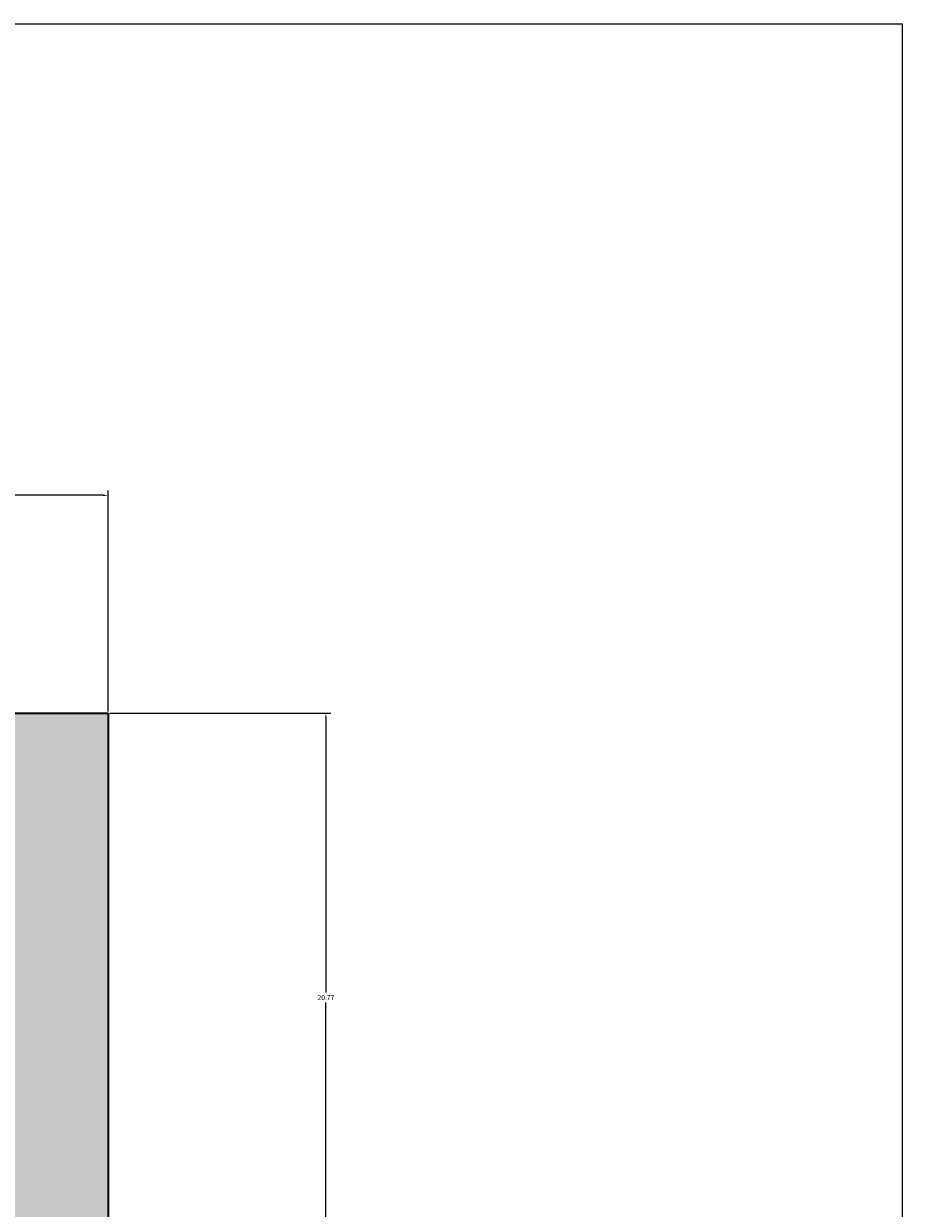
# Model space of a CAD drawing. Units: inches. Extents: x 4508 to 4723, y 847 to 1020.
# Tile 32 of 32: x 4691 to 4723, y 977 to 1020. Entities that reach past the tile are written whole.
import ezdxf

# ---------------------------------------------------------------- set-up
doc = ezdxf.new("R2010")
doc.units = ezdxf.units.IN
for name, color, linetype, lineweight in [('A-ANNO-DIMS', 2, 'Continuous', 18), ('A-ANNO-TTLB', 7, 'Continuous', 25), ('A-WALL', 7, 'Continuous', 35), ('A-WALL-PATT', 254, 'Continuous', 13)]:
    doc.layers.add(name, color=color, linetype=linetype, lineweight=lineweight)
doc.styles.get("Standard").update_dxf_attribs({"font": 'arial.ttf'})
doc.dimstyles.get("Standard").update_dxf_attribs({"dimtxt": 0.18, "dimasz": 0.18, "dimexe": 0.18, "dimexo": 0.0625, "dimgap": 0.09, "dimtad": 0, "dimtih": 1, "dimtoh": 1, "dimdec": 4, "dimzin": 0, "dimdsep": 46, "dimtxsty": 'Standard', "dimcen": 0.09, "dimadec": 0, "dimazin": 0, "dimtfac": 1, "dimtdec": 4, "dimtofl": 0, "dimtmove": 0, "dimatfit": 3, "dimfxl": 1, "dimtolj": 1, "dimtzin": 0, "dimarcsym": 0})

# ---------------------------------------------------------------- blocks, each defined once
blk = doc.blocks.new('*D11')
at = {"layer": 'A-ANNO-DIMS', "color": 0, "lineweight": -2, "transparency": 16777216}
for p, q in [((4671.806, 994.809), (4671.806, 1002.877)), ((4693.994, 994.809), (4693.994, 1002.877)), ((4671.986, 1002.697), (4682.435, 1002.697)), ((4693.814, 1002.697), (4683.365, 1002.697))]:
    blk.add_line(p, q, dxfattribs=at)
at = {"layer": 'A-ANNO-DIMS', "color": 0, "lineweight": 9, "transparency": 16777216}
for points in [[(4671.986, 1002.727), (4671.986, 1002.667), (4671.806, 1002.697)], [(4693.814, 1002.727), (4693.814, 1002.667), (4693.994, 1002.697)]]:
    blk.add_solid(points, dxfattribs=at)
at = {"layer": 'Defpoints', "color": 0, "lineweight": 9, "transparency": 16777216}
for p in [(4693.994, 1002.697), (4671.806, 994.747), (4693.994, 994.747)]:
    blk.add_point(p, dxfattribs=at)
at = {"layer": 'A-ANNO-DIMS', "color": 0, "transparency": 16777216, "insert": (4682.9, 1002.697), "char_height": 0.18, "attachment_point": 5}
blk.add_mtext('\\A1;22.188', dxfattribs=at)
blk = doc.blocks.new('*D23')
at = {"layer": 'A-ANNO-DIMS', "color": 0, "lineweight": -2, "transparency": 16777216}
for p, q in [((4694.056, 994.747), (4702.124, 994.747)), ((4701.944, 994.567), (4701.944, 984.545)), ((4701.944, 974.158), (4701.944, 984.181)), ((4669.387, 973.978), (4702.124, 973.978))]:
    blk.add_line(p, q, dxfattribs=at)
at = {"layer": 'A-ANNO-DIMS', "color": 0, "lineweight": 9, "transparency": 16777216}
for points in [[(4701.914, 994.567), (4701.974, 994.567), (4701.944, 994.747)], [(4701.914, 974.158), (4701.974, 974.158), (4701.944, 973.978)]]:
    blk.add_solid(points, dxfattribs=at)
at = {"layer": 'Defpoints', "color": 0, "lineweight": 9, "transparency": 16777216}
for p in [(4693.994, 994.747), (4701.944, 994.747), (4669.325, 973.978)]:
    blk.add_point(p, dxfattribs=at)
at = {"layer": 'A-ANNO-DIMS', "color": 0, "transparency": 16777216, "insert": (4701.944, 984.363), "char_height": 0.18, "attachment_point": 5}
blk.add_mtext('\\A1;20.77', dxfattribs=at)

msp = doc.modelspace()

# ---------------------------------------------------------------- hatches: boundary and pattern name
at = {"layer": 'A-WALL-PATT', "transparency": 33554508}
h = msp.add_hatch(color=256, dxfattribs=at)
h.dxf.hatch_style = 1
h.paths.add_polyline_path([(4661.6706, 954.043, -0.3739004), (4658.5765, 957.6021, -1), (4665.7646, 957.6021, -0.3739004), (4662.6706, 954.043), (4662.6706, 944.4021, -0.2114781), (4670.3062, 945.0869), (4670.3062, 968.0592, -0.4632086), (4663.3246, 973.9783, -0.4632086), (4670.3062, 979.8975), (4670.3062, 994.7469), (4588.9938, 994.7469), (4588.9938, 904.7469), (4657.9938, 904.7469), (4657.9938, 886.7469), (4549.9938, 886.7469), (4549.9938, 878.7469), (4693.9938, 878.7469), (4693.9938, 994.7469), (4671.8062, 994.7469), (4671.8062, 979.4411, -0.2941682), (4675.3246, 973.9783, -0.2941682), (4671.8062, 968.5156), (4671.8062, 944.4278, -0.2741114), (4676.7298, 936.1217, -0.2741114), (4671.8062, 927.8155), (4671.8062, 907.6998, -0.3779645), (4677.0562, 901.7469, -0.3779645), (4671.8062, 895.7939), (4671.8062, 883.7469), (4670.3062, 883.7469), (4670.3062, 895.7939, -0.3779645), (4665.0562, 901.7469, -0.3779645), (4670.3062, 907.6998), (4670.3062, 927.1564, -0.2114781), (4662.6706, 927.8412), (4662.6706, 918.2003, -0.3739004), (4665.7646, 914.6412, -1), (4658.5765, 914.6412, -0.3739004), (4661.6706, 918.2003), (4661.6706, 928.4807, -0.2391825), (4657.7936, 936.1217, -0.2391825), (4661.6706, 943.7626)])

# ---------------------------------------------------------------- linework, layer by layer
at = {"layer": 'A-ANNO-TTLB'}
msp.add_lwpolyline([(4508.3867, 1019.9118), (4722.9774, 1019.9118), (4722.9774, 846.9535), (4508.3867, 846.9535)], close=True, dxfattribs=at)
at = {"layer": 'A-WALL'}
for p, q in [((4540.9938, 994.7469), (4693.9938, 994.7469)), ((4693.9938, 994.7469), (4693.9938, 874.7469))]:
    msp.add_line(p, q, dxfattribs=at)

# ---------------------------------------------------------------- dimensions: what is measured, and where the dimension line sits
at = {"layer": 'A-ANNO-DIMS'}
dim = msp.add_linear_dim(base=(4693.9938, 1002.6969), p1=(4671.8062, 994.7469), p2=(4693.9938, 994.7469), dimstyle='Standard', override={"dimdec": 3, "dimlfac": 1, "dimrnd": 0, "dimzin": 0, "dimdsep": 46, "dimlunit": 2}, dxfattribs=at)
dim.commit()
dim.dimension.update_dxf_attribs({"geometry": '*D11', "text_midpoint": (4682.9, 1002.6969)})
dim = msp.add_linear_dim(base=(4701.9438, 994.7469), p1=(4669.3246, 973.9783), p2=(4693.9938, 994.7469), angle=90, dimstyle='Standard', override={"dimdec": 2, "dimlfac": 1, "dimrnd": 0, "dimzin": 0, "dimdsep": 46, "dimlunit": 2}, dxfattribs=at)
dim.commit()
dim.dimension.update_dxf_attribs({"geometry": '*D23', "text_midpoint": (4701.9438, 984.3626)})

doc.saveas('drawing.dxf')
